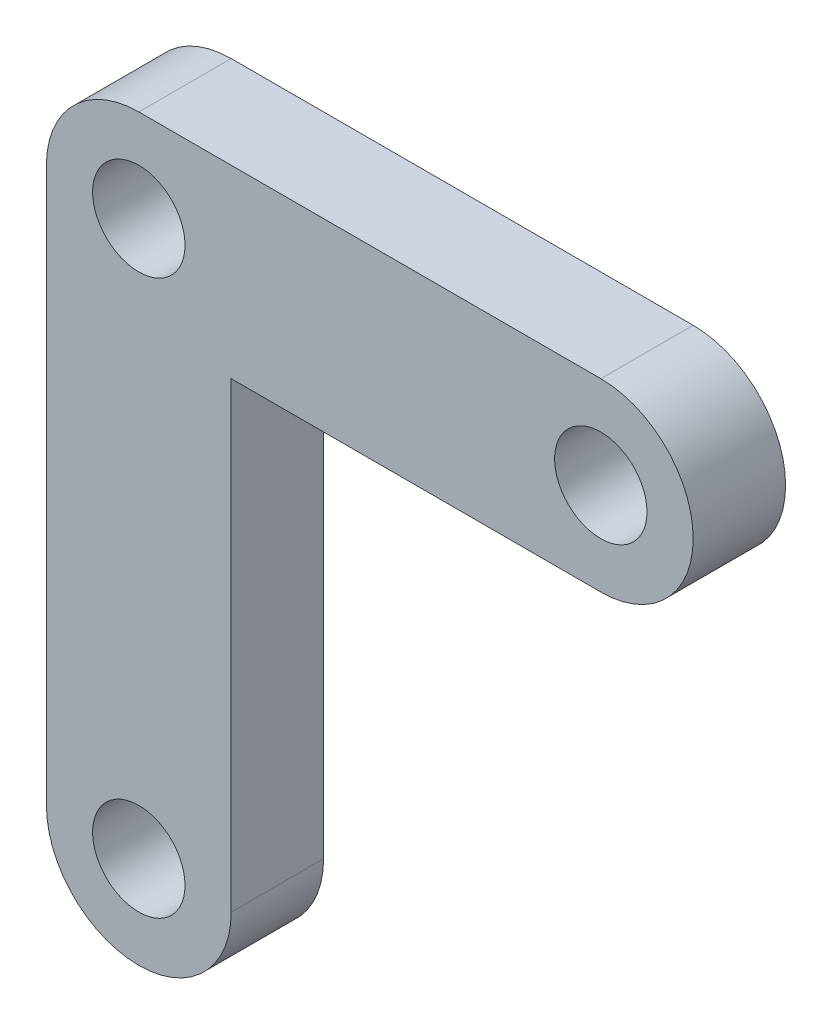
ISO-10303-21;
HEADER;
FILE_DESCRIPTION(('STEP AP214'),'2;1');
FILE_NAME('part.step','',(''),(''),'','','');
FILE_SCHEMA(('AUTOMOTIVE_DESIGN { 1 0 10303 214 1 1 1 1 }'));
ENDSEC;
DATA;
#1=APPLICATION_CONTEXT('core data for automotive mechanical design processes');
#2=APPLICATION_PROTOCOL_DEFINITION('international standard','automotive_design',2000,#1);
#3=PRODUCT_CONTEXT('',#1,'mechanical');
#4=PRODUCT('Part','Part','',(#3));
#5=PRODUCT_RELATED_PRODUCT_CATEGORY('part','',(#4));
#6=PRODUCT_DEFINITION_FORMATION('','',#4);
#7=PRODUCT_DEFINITION_CONTEXT('part definition',#1,'design');
#8=PRODUCT_DEFINITION('design','',#6,#7);
#9=PRODUCT_DEFINITION_SHAPE('','',#8);
#10=(LENGTH_UNIT() NAMED_UNIT(*) SI_UNIT(.MILLI.,.METRE.));
#11=(NAMED_UNIT(*) PLANE_ANGLE_UNIT() SI_UNIT($,.RADIAN.));
#12=(NAMED_UNIT(*) SI_UNIT($,.STERADIAN.) SOLID_ANGLE_UNIT());
#13=UNCERTAINTY_MEASURE_WITH_UNIT(LENGTH_MEASURE(1.E-05),#10,'distance_accuracy_value','');
#14=(GEOMETRIC_REPRESENTATION_CONTEXT(3) GLOBAL_UNCERTAINTY_ASSIGNED_CONTEXT((#13)) GLOBAL_UNIT_ASSIGNED_CONTEXT((#10,
#11,#12)) REPRESENTATION_CONTEXT('',''));
#15=CARTESIAN_POINT('',(0.,0.,0.));
#16=DIRECTION('',(0.,0.,1.));
#17=DIRECTION('',(1.,0.,0.));
#18=AXIS2_PLACEMENT_3D('',#15,#16,#17);
#19=CARTESIAN_POINT('',(0.,5.,5.));
#20=DIRECTION('',(0.,1.,0.));
#21=DIRECTION('',(0.,0.,1.));
#22=AXIS2_PLACEMENT_3D('',#19,#20,#21);
#23=PLANE('',#22);
#24=DIRECTION('',(1.,0.,0.));
#25=VECTOR('',#24,1.);
#26=CARTESIAN_POINT('',(0.,5.,0.));
#27=LINE('',#26,#25);
#28=CARTESIAN_POINT('',(0.,5.,0.));
#29=VERTEX_POINT('',#28);
#30=CARTESIAN_POINT('',(25.,5.,0.));
#31=VERTEX_POINT('',#30);
#32=EDGE_CURVE('E138',#29,#31,#27,.T.);
#33=ORIENTED_EDGE('',*,*,#32,.F.);
#34=DIRECTION('',(0.,0.,-1.));
#35=VECTOR('',#34,1.);
#36=CARTESIAN_POINT('',(0.,5.,5.));
#37=LINE('',#36,#35);
#38=CARTESIAN_POINT('',(0.,5.,5.));
#39=VERTEX_POINT('',#38);
#40=EDGE_CURVE('E11',#39,#29,#37,.T.);
#41=ORIENTED_EDGE('',*,*,#40,.F.);
#42=DIRECTION('',(1.,0.,0.));
#43=VECTOR('',#42,1.);
#44=CARTESIAN_POINT('',(0.,5.,5.));
#45=LINE('',#44,#43);
#46=CARTESIAN_POINT('',(25.,5.,5.));
#47=VERTEX_POINT('',#46);
#48=EDGE_CURVE('E162',#39,#47,#45,.T.);
#49=ORIENTED_EDGE('',*,*,#48,.T.);
#50=DIRECTION('',(0.,0.,-1.));
#51=VECTOR('',#50,1.);
#52=CARTESIAN_POINT('',(25.,5.,5.));
#53=LINE('',#52,#51);
#54=EDGE_CURVE('E90',#47,#31,#53,.T.);
#55=ORIENTED_EDGE('',*,*,#54,.T.);
#56=EDGE_LOOP('',(#33,#41,#49,#55));
#57=FACE_BOUND('',#56,.T.);
#58=ADVANCED_FACE('F41',(#57),#23,.T.);
#59=CARTESIAN_POINT('',(0.,0.,5.));
#60=DIRECTION('',(0.,0.,-1.));
#61=DIRECTION('',(-1.,0.,0.));
#62=AXIS2_PLACEMENT_3D('',#59,#60,#61);
#63=CYLINDRICAL_SURFACE('',#62,5.);
#64=CARTESIAN_POINT('',(0.,0.,0.));
#65=DIRECTION('',(0.,0.,1.));
#66=DIRECTION('',(1.,0.,0.));
#67=AXIS2_PLACEMENT_3D('',#64,#65,#66);
#68=CIRCLE('',#67,5.);
#69=CARTESIAN_POINT('',(-5.,0.,0.));
#70=VERTEX_POINT('',#69);
#71=EDGE_CURVE('E142',#29,#70,#68,.T.);
#72=ORIENTED_EDGE('',*,*,#71,.T.);
#73=DIRECTION('',(0.,0.,-1.));
#74=VECTOR('',#73,1.);
#75=CARTESIAN_POINT('',(-5.,0.,5.));
#76=LINE('',#75,#74);
#77=CARTESIAN_POINT('',(-5.,0.,5.));
#78=VERTEX_POINT('',#77);
#79=EDGE_CURVE('E47',#78,#70,#76,.T.);
#80=ORIENTED_EDGE('',*,*,#79,.F.);
#81=CARTESIAN_POINT('',(0.,0.,5.));
#82=DIRECTION('',(0.,0.,1.));
#83=DIRECTION('',(1.,0.,0.));
#84=AXIS2_PLACEMENT_3D('',#81,#82,#83);
#85=CIRCLE('',#84,5.);
#86=EDGE_CURVE('E181',#39,#78,#85,.T.);
#87=ORIENTED_EDGE('',*,*,#86,.F.);
#88=ORIENTED_EDGE('',*,*,#40,.T.);
#89=EDGE_LOOP('',(#72,#80,#87,#88));
#90=FACE_BOUND('',#89,.T.);
#91=ADVANCED_FACE('F179',(#90),#63,.T.);
#92=CARTESIAN_POINT('',(-5.,0.,5.));
#93=DIRECTION('',(-1.,0.,0.));
#94=DIRECTION('',(0.,0.,1.));
#95=AXIS2_PLACEMENT_3D('',#92,#93,#94);
#96=PLANE('',#95);
#97=DIRECTION('',(0.,1.,0.));
#98=VECTOR('',#97,1.);
#99=CARTESIAN_POINT('',(-5.,0.,0.));
#100=LINE('',#99,#98);
#101=CARTESIAN_POINT('',(-5.,-30.,0.));
#102=VERTEX_POINT('',#101);
#103=EDGE_CURVE('E144',#102,#70,#100,.T.);
#104=ORIENTED_EDGE('',*,*,#103,.F.);
#105=DIRECTION('',(0.,0.,-1.));
#106=VECTOR('',#105,1.);
#107=CARTESIAN_POINT('',(-5.,-30.,5.));
#108=LINE('',#107,#106);
#109=CARTESIAN_POINT('',(-5.,-30.,5.));
#110=VERTEX_POINT('',#109);
#111=EDGE_CURVE('E170',#110,#102,#108,.T.);
#112=ORIENTED_EDGE('',*,*,#111,.F.);
#113=DIRECTION('',(0.,1.,0.));
#114=VECTOR('',#113,1.);
#115=CARTESIAN_POINT('',(-5.,0.,5.));
#116=LINE('',#115,#114);
#117=EDGE_CURVE('E174',#110,#78,#116,.T.);
#118=ORIENTED_EDGE('',*,*,#117,.T.);
#119=ORIENTED_EDGE('',*,*,#79,.T.);
#120=EDGE_LOOP('',(#104,#112,#118,#119));
#121=FACE_BOUND('',#120,.T.);
#122=ADVANCED_FACE('F175',(#121),#96,.T.);
#123=CARTESIAN_POINT('',(0.,-30.,5.));
#124=DIRECTION('',(0.,0.,-1.));
#125=DIRECTION('',(-1.,0.,0.));
#126=AXIS2_PLACEMENT_3D('',#123,#124,#125);
#127=CYLINDRICAL_SURFACE('',#126,5.);
#128=CARTESIAN_POINT('',(0.,-30.,0.));
#129=DIRECTION('',(0.,0.,1.));
#130=DIRECTION('',(1.,0.,0.));
#131=AXIS2_PLACEMENT_3D('',#128,#129,#130);
#132=CIRCLE('',#131,5.);
#133=CARTESIAN_POINT('',(5.,-30.,0.));
#134=VERTEX_POINT('',#133);
#135=EDGE_CURVE('E146',#102,#134,#132,.T.);
#136=ORIENTED_EDGE('',*,*,#135,.T.);
#137=DIRECTION('',(0.,0.,-1.));
#138=VECTOR('',#137,1.);
#139=CARTESIAN_POINT('',(5.,-30.,5.));
#140=LINE('',#139,#138);
#141=CARTESIAN_POINT('',(5.,-30.,5.));
#142=VERTEX_POINT('',#141);
#143=EDGE_CURVE('E121',#142,#134,#140,.T.);
#144=ORIENTED_EDGE('',*,*,#143,.F.);
#145=CARTESIAN_POINT('',(0.,-30.,5.));
#146=DIRECTION('',(0.,0.,1.));
#147=DIRECTION('',(1.,0.,0.));
#148=AXIS2_PLACEMENT_3D('',#145,#146,#147);
#149=CIRCLE('',#148,5.);
#150=EDGE_CURVE('E114',#110,#142,#149,.T.);
#151=ORIENTED_EDGE('',*,*,#150,.F.);
#152=ORIENTED_EDGE('',*,*,#111,.T.);
#153=EDGE_LOOP('',(#136,#144,#151,#152));
#154=FACE_BOUND('',#153,.T.);
#155=ADVANCED_FACE('F185',(#154),#127,.T.);
#156=CARTESIAN_POINT('',(5.,0.,5.));
#157=DIRECTION('',(-1.,0.,0.));
#158=DIRECTION('',(0.,0.,1.));
#159=AXIS2_PLACEMENT_3D('',#156,#157,#158);
#160=PLANE('',#159);
#161=DIRECTION('',(0.,1.,0.));
#162=VECTOR('',#161,1.);
#163=CARTESIAN_POINT('',(5.,0.,0.));
#164=LINE('',#163,#162);
#165=CARTESIAN_POINT('',(5.,-5.,0.));
#166=VERTEX_POINT('',#165);
#167=EDGE_CURVE('E124',#134,#166,#164,.T.);
#168=ORIENTED_EDGE('',*,*,#167,.T.);
#169=DIRECTION('',(0.,0.,-1.));
#170=VECTOR('',#169,1.);
#171=CARTESIAN_POINT('',(5.,-5.,5.));
#172=LINE('',#171,#170);
#173=CARTESIAN_POINT('',(5.,-5.,5.));
#174=VERTEX_POINT('',#173);
#175=EDGE_CURVE('E119',#174,#166,#172,.T.);
#176=ORIENTED_EDGE('',*,*,#175,.F.);
#177=DIRECTION('',(0.,1.,0.));
#178=VECTOR('',#177,1.);
#179=CARTESIAN_POINT('',(5.,0.,5.));
#180=LINE('',#179,#178);
#181=EDGE_CURVE('E104',#142,#174,#180,.T.);
#182=ORIENTED_EDGE('',*,*,#181,.F.);
#183=ORIENTED_EDGE('',*,*,#143,.T.);
#184=EDGE_LOOP('',(#168,#176,#182,#183));
#185=FACE_BOUND('',#184,.T.);
#186=ADVANCED_FACE('F116',(#185),#160,.F.);
#187=CARTESIAN_POINT('',(0.,-5.,5.));
#188=DIRECTION('',(0.,1.,0.));
#189=DIRECTION('',(0.,0.,1.));
#190=AXIS2_PLACEMENT_3D('',#187,#188,#189);
#191=PLANE('',#190);
#192=DIRECTION('',(1.,0.,0.));
#193=VECTOR('',#192,1.);
#194=CARTESIAN_POINT('',(0.,-5.,0.));
#195=LINE('',#194,#193);
#196=CARTESIAN_POINT('',(25.,-5.,0.));
#197=VERTEX_POINT('',#196);
#198=EDGE_CURVE('E81',#166,#197,#195,.T.);
#199=ORIENTED_EDGE('',*,*,#198,.T.);
#200=DIRECTION('',(0.,0.,-1.));
#201=VECTOR('',#200,1.);
#202=CARTESIAN_POINT('',(25.,-5.,5.));
#203=LINE('',#202,#201);
#204=CARTESIAN_POINT('',(25.,-5.,5.));
#205=VERTEX_POINT('',#204);
#206=EDGE_CURVE('E125',#205,#197,#203,.T.);
#207=ORIENTED_EDGE('',*,*,#206,.F.);
#208=DIRECTION('',(1.,0.,0.));
#209=VECTOR('',#208,1.);
#210=CARTESIAN_POINT('',(0.,-5.,5.));
#211=LINE('',#210,#209);
#212=EDGE_CURVE('E109',#174,#205,#211,.T.);
#213=ORIENTED_EDGE('',*,*,#212,.F.);
#214=ORIENTED_EDGE('',*,*,#175,.T.);
#215=EDGE_LOOP('',(#199,#207,#213,#214));
#216=FACE_BOUND('',#215,.T.);
#217=ADVANCED_FACE('F122',(#216),#191,.F.);
#218=CARTESIAN_POINT('',(0.,0.,5.));
#219=DIRECTION('',(0.,0.,-1.));
#220=DIRECTION('',(-1.,0.,0.));
#221=AXIS2_PLACEMENT_3D('',#218,#219,#220);
#222=CYLINDRICAL_SURFACE('',#221,2.5);
#223=CARTESIAN_POINT('',(0.,0.,5.));
#224=DIRECTION('',(0.,0.,1.));
#225=DIRECTION('',(1.,0.,0.));
#226=AXIS2_PLACEMENT_3D('',#223,#224,#225);
#227=CIRCLE('',#226,2.5);
#228=CARTESIAN_POINT('',(2.5,0.,5.));
#229=VERTEX_POINT('',#228);
#230=EDGE_CURVE('E134',#229,#229,#227,.T.);
#231=ORIENTED_EDGE('',*,*,#230,.T.);
#232=EDGE_LOOP('',(#231));
#233=FACE_BOUND('',#232,.T.);
#234=CARTESIAN_POINT('',(0.,0.,0.));
#235=DIRECTION('',(0.,0.,1.));
#236=DIRECTION('',(1.,0.,0.));
#237=AXIS2_PLACEMENT_3D('',#234,#235,#236);
#238=CIRCLE('',#237,2.5);
#239=CARTESIAN_POINT('',(2.5,0.,0.));
#240=VERTEX_POINT('',#239);
#241=EDGE_CURVE('E160',#240,#240,#238,.T.);
#242=ORIENTED_EDGE('',*,*,#241,.F.);
#243=EDGE_LOOP('',(#242));
#244=FACE_BOUND('',#243,.T.);
#245=ADVANCED_FACE('F205',(#233,#244),#222,.F.);
#246=CARTESIAN_POINT('',(25.,0.,5.));
#247=DIRECTION('',(0.,0.,-1.));
#248=DIRECTION('',(-1.,0.,0.));
#249=AXIS2_PLACEMENT_3D('',#246,#247,#248);
#250=CYLINDRICAL_SURFACE('',#249,2.5);
#251=CARTESIAN_POINT('',(25.,0.,5.));
#252=DIRECTION('',(0.,0.,1.));
#253=DIRECTION('',(1.,0.,0.));
#254=AXIS2_PLACEMENT_3D('',#251,#252,#253);
#255=CIRCLE('',#254,2.5);
#256=CARTESIAN_POINT('',(27.5,0.,5.));
#257=VERTEX_POINT('',#256);
#258=EDGE_CURVE('E130',#257,#257,#255,.T.);
#259=ORIENTED_EDGE('',*,*,#258,.T.);
#260=EDGE_LOOP('',(#259));
#261=FACE_BOUND('',#260,.T.);
#262=CARTESIAN_POINT('',(25.,0.,0.));
#263=DIRECTION('',(0.,0.,1.));
#264=DIRECTION('',(1.,0.,0.));
#265=AXIS2_PLACEMENT_3D('',#262,#263,#264);
#266=CIRCLE('',#265,2.5);
#267=CARTESIAN_POINT('',(27.5,0.,0.));
#268=VERTEX_POINT('',#267);
#269=EDGE_CURVE('E152',#268,#268,#266,.T.);
#270=ORIENTED_EDGE('',*,*,#269,.F.);
#271=EDGE_LOOP('',(#270));
#272=FACE_BOUND('',#271,.T.);
#273=ADVANCED_FACE('F210',(#261,#272),#250,.F.);
#274=CARTESIAN_POINT('',(25.,0.,5.));
#275=DIRECTION('',(0.,0.,-1.));
#276=DIRECTION('',(-1.,0.,0.));
#277=AXIS2_PLACEMENT_3D('',#274,#275,#276);
#278=CYLINDRICAL_SURFACE('',#277,5.);
#279=CARTESIAN_POINT('',(25.,0.,0.));
#280=DIRECTION('',(0.,0.,1.));
#281=DIRECTION('',(1.,0.,0.));
#282=AXIS2_PLACEMENT_3D('',#279,#280,#281);
#283=CIRCLE('',#282,5.);
#284=EDGE_CURVE('E155',#197,#31,#283,.T.);
#285=ORIENTED_EDGE('',*,*,#284,.T.);
#286=ORIENTED_EDGE('',*,*,#54,.F.);
#287=CARTESIAN_POINT('',(25.,0.,5.));
#288=DIRECTION('',(0.,0.,1.));
#289=DIRECTION('',(1.,0.,0.));
#290=AXIS2_PLACEMENT_3D('',#287,#288,#289);
#291=CIRCLE('',#290,5.);
#292=EDGE_CURVE('E60',#205,#47,#291,.T.);
#293=ORIENTED_EDGE('',*,*,#292,.F.);
#294=ORIENTED_EDGE('',*,*,#206,.T.);
#295=EDGE_LOOP('',(#285,#286,#293,#294));
#296=FACE_BOUND('',#295,.T.);
#297=ADVANCED_FACE('F201',(#296),#278,.T.);
#298=CARTESIAN_POINT('',(0.,-30.,5.));
#299=DIRECTION('',(0.,0.,-1.));
#300=DIRECTION('',(-1.,0.,0.));
#301=AXIS2_PLACEMENT_3D('',#298,#299,#300);
#302=CYLINDRICAL_SURFACE('',#301,2.5);
#303=CARTESIAN_POINT('',(0.,-30.,5.));
#304=DIRECTION('',(0.,0.,1.));
#305=DIRECTION('',(1.,0.,0.));
#306=AXIS2_PLACEMENT_3D('',#303,#304,#305);
#307=CIRCLE('',#306,2.5);
#308=CARTESIAN_POINT('',(2.5,-30.,5.));
#309=VERTEX_POINT('',#308);
#310=EDGE_CURVE('E139',#309,#309,#307,.T.);
#311=ORIENTED_EDGE('',*,*,#310,.T.);
#312=EDGE_LOOP('',(#311));
#313=FACE_BOUND('',#312,.T.);
#314=CARTESIAN_POINT('',(0.,-30.,0.));
#315=DIRECTION('',(0.,0.,1.));
#316=DIRECTION('',(1.,0.,0.));
#317=AXIS2_PLACEMENT_3D('',#314,#315,#316);
#318=CIRCLE('',#317,2.5);
#319=CARTESIAN_POINT('',(2.5,-30.,0.));
#320=VERTEX_POINT('',#319);
#321=EDGE_CURVE('E159',#320,#320,#318,.T.);
#322=ORIENTED_EDGE('',*,*,#321,.F.);
#323=EDGE_LOOP('',(#322));
#324=FACE_BOUND('',#323,.T.);
#325=ADVANCED_FACE('F206',(#313,#324),#302,.F.);
#326=CARTESIAN_POINT('',(0.,0.,5.));
#327=DIRECTION('',(0.,0.,1.));
#328=DIRECTION('',(1.,0.,0.));
#329=AXIS2_PLACEMENT_3D('',#326,#327,#328);
#330=PLANE('',#329);
#331=ORIENTED_EDGE('',*,*,#48,.F.);
#332=ORIENTED_EDGE('',*,*,#86,.T.);
#333=ORIENTED_EDGE('',*,*,#117,.F.);
#334=ORIENTED_EDGE('',*,*,#150,.T.);
#335=ORIENTED_EDGE('',*,*,#181,.T.);
#336=ORIENTED_EDGE('',*,*,#212,.T.);
#337=ORIENTED_EDGE('',*,*,#292,.T.);
#338=EDGE_LOOP('',(#331,#332,#333,#334,#335,#336,#337));
#339=FACE_BOUND('',#338,.T.);
#340=ORIENTED_EDGE('',*,*,#258,.F.);
#341=EDGE_LOOP('',(#340));
#342=FACE_BOUND('',#341,.T.);
#343=ORIENTED_EDGE('',*,*,#230,.F.);
#344=EDGE_LOOP('',(#343));
#345=FACE_BOUND('',#344,.T.);
#346=ORIENTED_EDGE('',*,*,#310,.F.);
#347=EDGE_LOOP('',(#346));
#348=FACE_BOUND('',#347,.T.);
#349=ADVANCED_FACE('F110',(#339,#342,#345,#348),#330,.T.);
#350=CARTESIAN_POINT('',(0.,0.,0.));
#351=DIRECTION('',(0.,0.,1.));
#352=DIRECTION('',(1.,0.,0.));
#353=AXIS2_PLACEMENT_3D('',#350,#351,#352);
#354=PLANE('',#353);
#355=ORIENTED_EDGE('',*,*,#32,.T.);
#356=ORIENTED_EDGE('',*,*,#284,.F.);
#357=ORIENTED_EDGE('',*,*,#198,.F.);
#358=ORIENTED_EDGE('',*,*,#167,.F.);
#359=ORIENTED_EDGE('',*,*,#135,.F.);
#360=ORIENTED_EDGE('',*,*,#103,.T.);
#361=ORIENTED_EDGE('',*,*,#71,.F.);
#362=EDGE_LOOP('',(#355,#356,#357,#358,#359,#360,#361));
#363=FACE_BOUND('',#362,.T.);
#364=ORIENTED_EDGE('',*,*,#269,.T.);
#365=EDGE_LOOP('',(#364));
#366=FACE_BOUND('',#365,.T.);
#367=ORIENTED_EDGE('',*,*,#241,.T.);
#368=EDGE_LOOP('',(#367));
#369=FACE_BOUND('',#368,.T.);
#370=ORIENTED_EDGE('',*,*,#321,.T.);
#371=EDGE_LOOP('',(#370));
#372=FACE_BOUND('',#371,.T.);
#373=ADVANCED_FACE('F178',(#363,#366,#369,#372),#354,.F.);
#374=CLOSED_SHELL('',(#58,#91,#122,#155,#186,#217,#245,#273,#297,#325,#349,#373));
#375=MANIFOLD_SOLID_BREP('B2',#374);
#376=ADVANCED_BREP_SHAPE_REPRESENTATION('',(#18,#375),#14);
#377=SHAPE_DEFINITION_REPRESENTATION(#9,#376);
ENDSEC;
END-ISO-10303-21;
